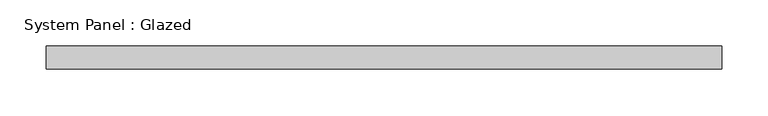
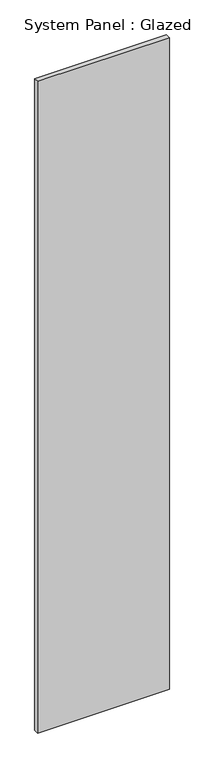
"""IFC4 building model written with IfcOpenShell, lengths in millimetres: plate geometry, System Panel : Glazed."""

from ifc_helpers import new_model, si_unit, origin, origin_with_axes, place, context, project, spatial, polyline, outline, extrude, source, transform, mapped, element, save


def system_panel_glazed_5544ac81(model_context):
    return source(origin(), model_context, "Body", "SweptSolid", [
        extrude(outline(polyline([(367.2009013, 19.05), (-367.2009013, 19.05), (-367.2009013, 44.45), (367.2009013, 44.45), (367.2009013, 19.05)])), origin_with_axes(), (0.0, 0.0, 1.0), 3833.0609328),
    ])


if __name__ == "__main__":
    model = new_model("IFC4")
    model_context = context("Model", 3, world=origin())
    ifc_project = project(units=[si_unit("LENGTHUNIT", "METRE", prefix="MILLI")], contexts=[model_context])
    site = spatial("IfcSite", under=ifc_project)
    building = spatial("IfcBuilding", under=site)
    placement = place(None, origin())
    system_panel_glazed_shape = system_panel_glazed_5544ac81(model_context)
    element("IfcPlate", 1, ObjectType="System Panel : Glazed", at=placement, inside=building, context=model_context, shape_type="MappedRepresentation", body=[
        mapped(system_panel_glazed_shape, transform((0.0, 0.0, 0.0), x_axis=(1.0, 0.0, 0.0), y_axis=(0.0, 1.0, 0.0), z_axis=(0.0, 0.0, 1.0))),
    ])
    save(model, "model.ifc")

# Revit data of these elements
# Type "System Panel : Glazed"
#   Construction Type Id = "GSP4R"
#   Analytic Construction = "1/8 in Pilkington single glazing"
#   Visual Light Transmittance = 0.9
#   Solar Heat Gain Coefficient = 0.86
#   Heat Transfer Coefficient (U) = 1.18115 BTU/(h·ft²·°F)
#   Define Thermal Properties by = 1
# Element 1 (IfcPlate, "System Panel : Glazed")
#   Materials on its faces: "Glass"
# Materials
#   "Glass": class "Glass", colour RGB 0 128 192, transparency 0.75, Description = "Soda Lime Glass", Cost = 0
